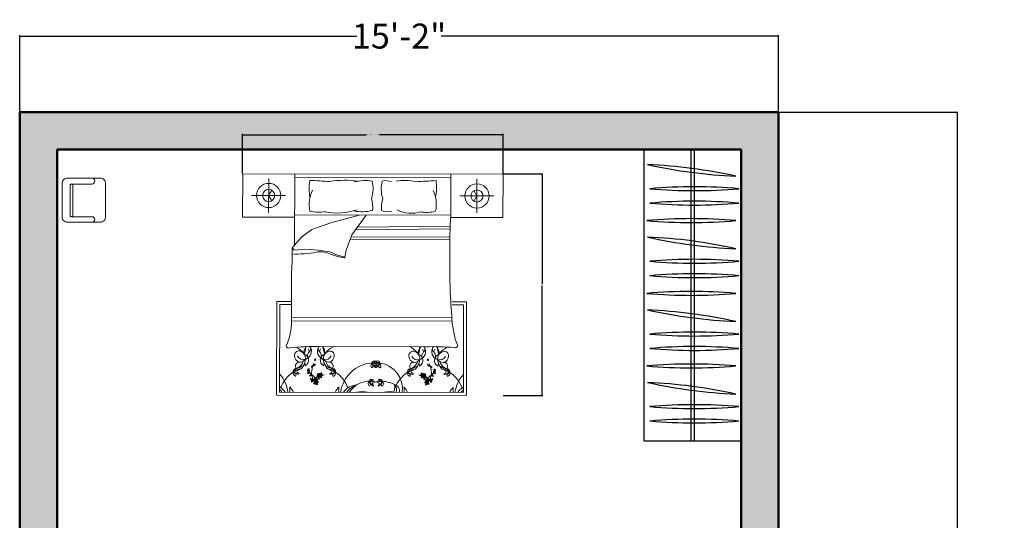
# Model space of a CAD drawing. Units: inches. Extents: x 3 to 485, y -522 to 42.
# Tile 6 of 6: x 249 to 485, y -84 to 36. Entities that reach past the tile are written whole.
import ezdxf

# ---------------------------------------------------------------- set-up
doc = ezdxf.new("R2010")
doc.units = ezdxf.units.IN
doc.header["$MEASUREMENT"] = 0
for name, color, linetype, lineweight in [('A-ANNO-DIMS', 2, 'Continuous', 18), ('A-FLOR-CASE', 8, 'Continuous', 25), ('A-FURN', 8, 'Continuous', 18), ('A-WALL', 7, 'Continuous', 50)]:
    doc.layers.add(name, color=color, linetype=linetype, lineweight=lineweight)
doc.layers.add('A-WALL-PATT', color=18, linetype='Continuous', lineweight=13, true_color=0x000000)
doc.styles.get("Standard").update_dxf_attribs({"font": 'arial.ttf'})
doc.dimstyles.get("Standard").update_dxf_attribs({"dimtxt": 0.18, "dimasz": 0.18, "dimexe": 0.18, "dimexo": 0.0625, "dimgap": 0.09, "dimtad": 0, "dimtih": 1, "dimtoh": 1, "dimdec": 0, "dimzin": 0, "dimdsep": 46, "dimlunit": 3, "dimtxsty": 'Standard', "dimcen": 0.09, "dimadec": 0, "dimazin": 0, "dimtfac": 1, "dimtdec": 0, "dimtofl": 0, "dimtmove": 0, "dimatfit": 3, "dimfxl": 1, "dimtolj": 1, "dimtzin": 0, "dimarcsym": 0})

# ---------------------------------------------------------------- blocks, each defined once
blk = doc.blocks.new('*D6')
at = {"layer": 'A-ANNO-DIMS', "color": 0, "lineweight": -2, "transparency": 16777216}
for p, q in [((248.79, 14.07), (248.79, 32.43)), ((248.97, 32.25), (329.68, 32.25)), ((430.61, 32.25), (349.9, 32.25)), ((430.79, 14.07), (430.79, 32.43))]:
    blk.add_line(p, q, dxfattribs=at)
at = {"layer": 'A-ANNO-DIMS', "color": 0, "transparency": 16777216}
for points in [[(248.97, 32.28), (248.97, 32.22), (248.79, 32.25)], [(430.61, 32.28), (430.61, 32.22), (430.79, 32.25)]]:
    blk.add_solid(points, dxfattribs=at)
at = {"layer": 'Defpoints', "color": 0, "transparency": 16777216}
for p in [(430.79, 32.25), (248.79, 14), (430.79, 14)]:
    blk.add_point(p, dxfattribs=at)
at = {"layer": 'A-ANNO-DIMS', "color": 0, "transparency": 16777216, "insert": (339.79, 32.25), "char_height": 6, "attachment_point": 5}
blk.add_mtext('\\A1;15\'-2"', dxfattribs=at)
blk = doc.blocks.new('*D7')
at = {"layer": 'A-ANNO-DIMS', "color": 0, "lineweight": -2, "transparency": 16777216}
for p, q in [((430.85, 14), (473.81, 14)), ((473.63, 13.82), (473.63, -230.89)), ((473.63, -481.82), (473.63, -237.1)), ((430.85, -482), (473.81, -482))]:
    blk.add_line(p, q, dxfattribs=at)
at = {"layer": 'A-ANNO-DIMS', "color": 0, "transparency": 16777216}
for points in [[(473.6, 13.82), (473.66, 13.82), (473.63, 14)], [(473.6, -481.82), (473.66, -481.82), (473.63, -482)]]:
    blk.add_solid(points, dxfattribs=at)
at = {"layer": 'Defpoints', "color": 0, "transparency": 16777216}
for p in [(430.79, 14), (430.79, -482), (473.63, -482)]:
    blk.add_point(p, dxfattribs=at)
at = {"layer": 'A-ANNO-DIMS', "color": 0, "transparency": 16777216, "insert": (473.63, -234), "char_height": 6, "attachment_point": 5}
blk.add_mtext('\\A1;41\'-4"', dxfattribs=at)
blk = doc.blocks.new('BED-DOUBLE-WITH-NIGHTSTANDS')
for p, q in [((53.23, 62.45), (53.09, 0)), ((48, 52.14), (48.02, 60.3)), ((0, 8.8), (0.1, 54.33)), ((0.1, 54.33), (22.6, 54.28)), ((43.93, 56.23), (52.09, 56.21)), ((0.82, 53.6), (0.73, 9.52)), ((21.87, 53.56), (0.82, 53.6)), ((21.87, 50.75), (21.87, 53.56)), ((22.6, 54.28), (22.59, 50.74)), ((17.83, 12.23), (17.92, 50.76)), ((18.61, 12.28), (18.7, 50.76)), ((34.9, 50.06), (35.41, 50.56)), ((35.15, 47.53), (34.9, 50.06)), ((35.41, 50.56), (38.06, 48.28)), ((53.2, 49.96), (36.06, 50)), ((43.33, 49.98), (43.25, 12.51)), ((52.32, 12.49), (52.4, 49.96)), ((7.14, 47.43), (7.85, 47.57)), ((34.89, 44.36), (35.15, 47.53)), ((38.06, 48.28), (39.83, 45.87)), ((39.83, 45.87), (41.46, 41.31)), ((7.13, 43.07), (7.84, 42.93)), ((11.71, 18.64), (11.77, 44)), ((34.51, 41.58), (34.89, 44.36)), ((33.74, 39.94), (34.51, 41.58)), ((41.46, 41.31), (43.3, 34.5)), ((33.23, 37.92), (33.74, 39.94)), ((34.88, 37.66), (33.23, 37.92)), ((38.54, 36.26), (34.88, 37.66)), ((37.41, 12.75), (37.36, 36.71)), ((38.05, 12.75), (38.01, 36.46)), ((43.3, 32.83), (38.54, 36.26)), ((40.02, 12.71), (39.75, 35.39)), ((40.66, 12.69), (40.39, 34.92)), ((7.08, 20.02), (7.79, 20.16)), ((7.07, 15.66), (7.78, 15.52)), ((21.78, 9.47), (21.78, 12.22)), ((22.51, 12.21), (22.5, 8.75)), ((0.73, 9.52), (21.78, 9.47)), ((47.91, 10.34), (47.89, 2.18)), ((22.5, 8.75), (0, 8.8)), ((43.82, 6.27), (51.98, 6.25))]:
    blk.add_line(p, q)
for points in [[(42.79, 49.99), (42.82, 62.48), (53.23, 62.45)], [(48.01, 56.22), (46.75, 55.49)], [(48.01, 56.22), (49.27, 55.49)], [(53.12, 12.49), (42.71, 12.51), (42.69, 0.02), (53.09, 0)], [(47.9, 6.26), (46.64, 6.99)], [(47.9, 6.26), (49.17, 6.98)]]:
    blk.add_lwpolyline(points)
for points in [[(29.69, 50.7, 0.001242), (17.84, 50.76, -0.127202), (11.94, 52.03)], [(51.64, 46.38, 0.074897), (47.56, 46.31, -0.472817)], [(47.3, 31.53, 0.14099), (51.46, 31.4, 0.235245)], [(47.29, 28.87, -0.14099), (51.46, 28.98, -0.235245)], [(51.57, 16.08, -0.074897), (47.49, 16.17, 0.472817)], [(19.1, 12.3, 0.056112), (15.67, 11.85, 0.095341), (12.35, 10.98)]]:
    blk.add_lwpolyline(points, format="xyb")
for centre, radius in [((48.01, 56.22), 2.91), ((48.01, 56.22), 1.46), ((3.2, 44.87), 0.159), ((4.87, 43.83), 0.159), ((4.82, 19.27), 0.159), ((3.14, 18.23), 0.159), ((47.9, 6.26), 2.91), ((47.9, 6.26), 1.46)]:
    blk.add_circle(centre, radius)
for centre, radius, start, end in [((-2.1, 57.02), 4.95, 306.1777, 316.3555), ((-1.36, 55.59), 3.97, 303.3358, 329.9857), ((-0.26, 59.68), 8.16, 277.6191, 311.7597), ((-1.1, 45.72), 8.16, 34.2606, 68.4649), ((11.98, 51.45), 0.576, 93.8541, 207.2153), ((-0.45, 53.36), 3.32, 292.4288, 318.8287), ((1.35, 62.44), 11.28, 267.2822, 273.526), ((5.45, 49.43), 0.904, 77.5856, 158.9128), ((4.96, 50.34), 0.681, 238.3374, 358.161), ((7.19, 48.96), 2.06, 138.7143, 177.8093), ((5.95, 49.72), 0.667, 117.5568, 223.6503), ((5.8, 49.66), 0.676, 2.8257, 103.6021), ((11.21, 51.54), 5.71, 192.3914, 207.0565), ((4.88, 49.27), 1.29, 345.3394, 54.1084), ((6.83, 51.04), 1.39, 211.2568, 255.171), ((7.09, 48.86), 0.937, 350.1381, 160.7429), ((9.5, 48.51), 1.49, 84.8189, 172.7598), ((9.65, 48.95), 1.05, 354.3597, 90.9279), ((-53.24, 44.88), 65.02, 359.2174, 5.5628), ((33.98, 107.83), 57.28, 265.7035, 271.4271), ((57.53, 49.44), 23.57, 177.326, 191.2133), ((5.23, 49.03), 0.101, 177.8093, 11.3575), ((5.28, 49.04), 0.0492, 11.3575, 127.815), ((5.53, 49.32), 0.0882, 223.6503, 159.5924), ((7.38, 49.09), 1.17, 175.8431, 254.1786), ((6.08, 49.06), 0.574, 333.8496, 53.1422), ((5.82, 47.83), 1.25, 6.0403, 51.4566), ((9.16, 50.72), 2.95, 211.1355, 251.5786), ((8.92, 50.74), 3.35, 236.1624, 266.3817), ((8.49, 48.2), 1.55, 209.7826, 343.0078), ((9.83, 48.77), 1.81, 182.2332, 233.9142), ((10.06, 47.93), 1.45, 111.456, 201.2962), ((8.87, 49.27), 1.88, 265.1674, 346.7951), ((9.14, 47.22), 0.388, 167.1782, 285.0212), ((10.18, 45.36), 2.41, 122.5752, 126.2186), ((10.64, 47.96), 1.99, 199.1563, 299.0492), ((11.32, 49.96), 2.59, 238.6959, 279.0295), ((10.18, 45.36), 2.41, 55.6591, 94.6045), ((7.39, 51.7), 4.73, 303.5412, 333.1738), ((11.08, 46.76), 0.752, 29.9034, 52.1991), ((2.9, 44.66), 0.263, 61.0937, 168.9144), ((3.07, 45.2), 0.314, 157.2827, 261.3127), ((2.9, 45.21), 0.158, 57.924, 135.5009), ((3.06, 45.11), 0.105, 172.7801, 277.0061), ((2.72, 44.92), 0.501, 14.6299, 57.924), ((3.42, 45.05), 0.217, 35.9787, 181.3022), ((3.43, 45.9), 0.178, 124.2279, 214.2664), ((3.69, 45.87), 0.414, 190.1798, 287.0699), ((3.29, 45.22), 0.219, 269.9386, 331.0248), ((3.48, 45.17), 0.25, 221.7153, 265.6618), ((3.81, 46.02), 0.481, 176.8442, 248.1654), ((7.25, 48.55), 4.65, 212.5525, 216.2487), ((3.48, 45.07), 0.156, 263.6267, 41.5794), ((3.44, 44.65), 0.265, 11.4378, 86.2391), ((3.65, 45.91), 0.184, 216.2487, 291.6289), ((5.27, 43.32), 2.59, 123.8774, 132.3658), ((2.6, 43), 2.77, 63.656, 68.1654), ((4.08, 45.13), 0.441, 128.1949, 208.6903), ((4.09, 45.78), 0.414, 122.6896, 187.2733), ((4.16, 45.16), 0.527, 207.5784, 254.2257), ((3.77, 45.61), 0.139, 289.2346, 111.6289), ((3.87, 45.61), 0.139, 221.7444, 44.1387), ((4.5, 45.2), 0.725, 157.1046, 228.9376), ((4.27, 45.72), 0.481, 109.354, 177.5569), ((4.25, 45.44), 0.427, 174.3285, 220.4929), ((1.82, 43.06), 3.11, 30.4181, 49.6921), ((4.01, 46.03), 0.178, 56.7377, 146.7762), ((4.1, 45.83), 0.184, 148.7585, 224.1387), ((3.54, 44.83), 0.513, 339.8782, 40.4929), ((7.92, 43.52), 4.65, 145.0623, 148.7585), ((5.27, 43.32), 2.59, 94.6301, 119.0782), ((10.78, 39.58), 8.53, 132.1153, 142.0485), ((6.49, 46.38), 1.76, 178.2005, 187.0043), ((4.59, 46.14), 0.328, 11.1997, 64.3362), ((5.7, 46.61), 0.987, 190.1329, 210.5301), ((5.04, 46.21), 0.3, 188.2173, 274.161), ((5.3, 46.37), 0.523, 210.5301, 242.5082), ((5.7, 46.82), 1, 218.0842, 226.1812), ((4.95, 45.98), 0.127, 325.6398, 67.3157), ((1.01, 50.24), 5.93, 313.0282, 321.92), ((5.39, 40.75), 5.17, 73.4583, 93.7018), ((5.37, 46.67), 0.122, 142.3478, 264.9271), ((5.53, 46.7), 0.263, 127.6362, 168.9144), ((5.39, 46.92), 0.37, 264.9271, 338.2359), ((5.88, 46.41), 0.483, 113.3017, 137.4845), ((5.82, 46.91), 0.159, 183.1509, 356.5973), ((5.94, 46.62), 0.26, 139.663, 227.5532), ((5.85, 46.53), 0.137, 227.5532, 350.2228), ((5.32, 46.63), 0.521, 352.9593, 15.5912), ((5.67, 46.57), 0.329, 350.2228, 43.5279), ((6.28, 46.9), 0.382, 198.6004, 262.3773), ((5.97, 46.73), 0.152, 0.9822, 91.7416), ((6.07, 46.69), 0.265, 11.4378, 52.5099), ((6.26, 46.64), 0.123, 255.1097, 54.7989), ((8.59, 46), 1.76, 178.2005, 187.0043), ((6.69, 45.76), 0.328, 11.1997, 64.3362), ((7.8, 46.23), 0.987, 190.1329, 210.5301), ((7.14, 45.83), 0.3, 188.2173, 274.161), ((7.4, 46), 0.523, 210.5301, 242.5082), ((7.8, 46.44), 1, 218.0842, 226.1812), ((7.05, 45.6), 0.127, 325.6398, 67.3157), ((7.41, 45.37), 0.3, 147.4073, 233.3509), ((7.68, 45.52), 0.523, 179.06, 211.0381), ((7.17, 45.41), 0.127, 354.2525, 95.9284), ((5.39, 40.75), 5.17, 62.8773, 69.7682), ((8.08, 45.76), 0.987, 211.0381, 231.4353), ((8.25, 46.56), 1.76, 234.5639, 243.3677), ((8.27, 45.66), 1, 195.387, 203.484), ((7.14, 45.01), 0.328, 357.232, 50.3685), ((8.55, 45.07), 0.12, 12.5792, 190.3125), ((8.62, 45.08), 0.196, 190.3125, 10.2877), ((9.57, 45.61), 1.28, 41.4394, 105.0212), ((10.28, 48.26), 1.8, 277.3101, 299.789), ((11.23, 47.07), 0.935, 221.4394, 293.7095), ((11.08, 46.76), 0.752, 314.3258, 333.4321), ((52.37, 44.15), 8.37, 164.978, 190.911), ((45.9, 38.43), 8.05, 65.0057, 101.6324), ((645.92, 10.65), 595.35, 176.55931, 177.02387), ((2.74, 44.63), 0.122, 142.3478, 264.9271), ((2.76, 44.88), 0.37, 264.9271, 338.2359), ((3.25, 44.37), 0.483, 113.3017, 137.4845), ((3.31, 44.59), 0.26, 139.663, 227.5532), ((3.23, 44.5), 0.137, 227.5532, 350.2228), ((2.7, 44.59), 0.521, 352.9593, 15.5912), ((3.04, 44.53), 0.329, 350.2228, 43.5279), ((3.65, 44.87), 0.382, 198.6004, 262.3773), ((3.35, 44.69), 0.152, 0.9822, 91.7416), ((3.63, 44.61), 0.123, 255.1097, 54.7989), ((3.82, 44.86), 0.725, 270.1521, 341.9851), ((4.3, 43.95), 0.513, 98.5968, 159.2116), ((4.05, 44.61), 0.527, 244.864, 291.5114), ((4.16, 44.88), 0.427, 278.5968, 324.7613), ((4.09, 44.54), 0.441, 290.3994, 358.4116), ((4.41, 43.59), 0.122, 142.3478, 264.9271), ((4.57, 43.61), 0.263, 61.0937, 168.9144), ((4.44, 43.84), 0.37, 264.9271, 338.2359), ((4.75, 44.15), 0.314, 157.2827, 261.3127), ((4.57, 44.17), 0.158, 57.924, 135.5009), ((4.95, 44.66), 0.441, 182.724, 265.9967), ((4.78, 44.97), 0.427, 231.6348, 277.7993), ((5.11, 45.05), 0.725, 214.411, 286.244), ((4.92, 43.33), 0.483, 113.3017, 137.4845), ((4.74, 44.07), 0.105, 172.7801, 277.0061), ((4.39, 43.87), 0.501, 14.6299, 57.924), ((1.82, 43.06), 3.11, 22.9242, 23.7218), ((4.99, 43.54), 0.26, 139.663, 227.5532), ((4.9, 43.45), 0.137, 227.5532, 350.2228), ((4.9, 44.04), 0.513, 37.1845, 97.7993), ((5.09, 44.01), 0.217, 35.9787, 181.3022), ((4.37, 43.55), 0.521, 352.9593, 15.5912), ((4.96, 44.75), 0.527, 264.8847, 311.5321), ((1.82, 43.06), 3.11, 356.9812, 4.6326), ((4.71, 43.48), 0.329, 350.2228, 43.5279), ((5.32, 43.82), 0.382, 198.6004, 262.3773), ((4.97, 44.18), 0.219, 269.9386, 331.0248), ((5.15, 44.12), 0.25, 221.7153, 265.6618), ((5.02, 43.64), 0.152, 0.9822, 91.7416), ((5.15, 44.03), 0.156, 263.6267, 41.5794), ((5.12, 43.61), 0.265, 11.4378, 86.2391), ((5.3, 43.56), 0.123, 255.1097, 54.7989), ((7.36, 41.41), 1.17, 105.5696, 183.9051), ((5.81, 42.68), 1.25, 308.2916, 353.7079), ((9.14, 39.78), 2.95, 108.1696, 148.6127), ((8.9, 39.75), 3.35, 93.3665, 123.5858), ((8.48, 42.29), 1.55, 16.7404, 149.9656), ((9.81, 41.72), 1.81, 125.834, 177.515), ((10.05, 42.56), 1.45, 158.4519, 248.2922), ((8.85, 41.22), 1.88, 12.9531, 94.5808), ((9.13, 43.27), 0.388, 74.727, 192.57), ((10.63, 42.53), 1.99, 60.699, 160.5919), ((10.18, 45.13), 2.41, 233.5296, 237.173), ((9.57, 44.88), 1.28, 254.727, 318.3088), ((11.3, 40.52), 2.59, 79.5874, 121.0523), ((10.18, 45.13), 2.41, 265.1437, 304.089), ((7.36, 38.8), 4.73, 21.3682, 56.207), ((10.27, 42.23), 1.8, 59.9592, 82.4381), ((11.22, 43.41), 0.935, 66.0387, 138.3088), ((11.08, 43.73), 0.752, 307.5491, 336.5885), ((11.08, 43.73), 0.752, 23.1031, 45.4224), ((29.42, 43.87), 5.08, 336.1357, 11.2133), ((58.3, 39.73), 14.52, 167.9138, 199.1356), ((-0.49, 37.18), 3.32, 40.9195, 67.3194), ((-1.1, 44.81), 8.16, 291.2833, 325.4876), ((4.94, 40.17), 0.681, 1.5872, 121.4108), ((5.43, 41.08), 0.904, 200.8354, 282.1626), ((5.21, 41.48), 0.101, 348.3907, 181.9389), ((7.17, 41.55), 2.06, 181.9389, 221.0339), ((5.26, 41.47), 0.0492, 231.9332, 348.3907), ((5.93, 40.78), 0.667, 136.0979, 242.1914), ((5.55, 41.17), 0.0532, 200.1408, 136.1012), ((4.87, 41.24), 1.29, 305.6398, 14.4087), ((11.19, 38.94), 5.71, 152.6917, 167.3568), ((5.78, 40.85), 0.676, 256.1461, 356.9225), ((6.81, 39.46), 1.39, 104.5772, 148.4914), ((7.08, 41.64), 0.937, 199.0053, 9.6101), ((6.06, 41.45), 0.574, 306.606, 25.8985), ((9.48, 41.98), 1.49, 186.9883, 274.9292), ((9.63, 41.55), 1.05, 268.8203, 5.3885), ((56.83, 33.53), 24.22, 159.9935, 169.2124), ((29.02, 37.87), 22.65, 352.0937, 9.3711), ((1.28, 28.09), 11.28, 86.2222, 92.466), ((-0.33, 30.86), 8.16, 4.3364, 82.1291), ((-1.41, 34.95), 3.97, 1.1461, 56.4124), ((33.18, 38.06), 0.151, 178.7364, 289.6277), ((-2.15, 33.52), 4.95, 17.7245, 53.5705), ((-3.55, 30.92), 7.37, 33.8864, 53.9271), ((55.12, 33.86), 11.01, 169.7358, 193.4979), ((40.46, 33.06), 11.13, 351.399, 13.8341), ((-3.51, 33.77), 4.48, 343.4172, 16.8943), ((-4.69, 31.49), 8.16, 4.3364, 27.2887), ((-5.82, 32), 6.63, 4.2528, 5.5098), ((-10.38, 28.52), 11.85, 19.5958, 19.7769), ((2.83, 31.44), 0.904, 47.6614, 128.9886), ((2.86, 32.47), 0.681, 208.4132, 328.2368), ((2.44, 31.2), 0.101, 147.8851, 341.4333), ((4.1, 30.16), 2.06, 108.79, 147.8851), ((2.49, 31.18), 0.0492, 341.4333, 97.8908), ((3.41, 31.44), 0.667, 87.6326, 193.7261), ((2.85, 31.31), 0.0882, 193.7261, 129.7986), ((8.88, 30.39), 5.71, 162.4671, 177.1323), ((2.26, 31.58), 1.29, 315.4152, 24.1842), ((4.83, 32.14), 1.39, 181.3326, 225.2468), ((3.25, 31.46), 0.676, 332.9015, 73.6778), ((7.2, 30.81), 0.904, 47.6614, 128.9886), ((7.23, 31.83), 0.681, 208.4132, 328.2368), ((8.47, 29.52), 2.06, 108.79, 147.8851), ((7.78, 30.81), 0.667, 87.6326, 193.7261), ((7.22, 30.67), 0.0882, 193.7261, 129.7986), ((6.63, 30.95), 1.29, 315.4152, 24.1842), ((13.25, 29.76), 5.71, 162.4671, 177.1323), ((6.63, 30.06), 1.29, 335.564, 44.333), ((13.25, 31.23), 5.71, 182.6159, 197.2811), ((7.62, 30.83), 0.676, 332.9015, 73.6778), ((9.2, 31.51), 1.39, 181.3326, 225.2468), ((45.23, 38.9), 7.65, 263.887, 285.7034), ((1.56, 30.44), 6.31, 262.7377, 351.6938), ((-3.52, 27.29), 4.48, 342.8539, 16.331), ((-5.83, 29.07), 6.63, 354.2384, 355.4954), ((-10.37, 32.57), 11.85, 339.9713, 340.1524), ((2.85, 28.56), 0.681, 31.5114, 151.335), ((2.83, 29.59), 0.904, 230.7596, 312.0868), ((2.44, 29.83), 0.101, 18.3149, 211.8631), ((4.1, 30.87), 2.06, 211.8631, 250.9581), ((2.49, 29.85), 0.0492, 261.8574, 18.3149), ((-4.7, 29.57), 8.16, 332.4595, 355.4118), ((3.41, 29.58), 0.667, 166.0221, 272.1156), ((2.88, 29.73), 0.0532, 230.065, 165.895), ((8.88, 30.61), 5.71, 182.6159, 197.2811), ((2.26, 29.45), 1.29, 335.564, 44.333), ((4.82, 28.88), 1.39, 134.5014, 178.4156), ((3.24, 29.57), 0.676, 286.0703, 26.8467), ((7.22, 29.18), 0.681, 31.5114, 151.335), ((7.2, 30.2), 0.904, 230.7596, 312.0868), ((6.81, 30.57), 0.101, 147.8851, 341.4333), ((6.81, 30.45), 0.101, 18.3149, 211.8631), ((8.47, 31.48), 2.06, 211.8631, 250.9581), ((6.86, 30.55), 0.0492, 341.4333, 97.8908), ((6.86, 30.46), 0.0492, 261.8574, 18.3149), ((7.78, 30.2), 0.667, 166.0221, 272.1156), ((7.25, 30.35), 0.0532, 230.065, 165.895), ((7.61, 30.18), 0.676, 286.0703, 26.8467), ((9.19, 29.49), 1.39, 134.5014, 178.4156), ((47.41, 27.72), 3.31, 154.8924, 198.4148), ((45.19, 21.51), 7.65, 74.0448, 95.8612), ((48.49, 28.13), 3.09, 333.2178, 15.9767), ((2.13, 29.63), 3.65, 247.9911, 276.4936), ((1.11, 26.28), 1.46, 256.2639, 348.9479), ((1.31, 27.38), 1.85, 252.735, 311.779), ((1.29, 35.03), 11.28, 267.2822, 273.526), ((-0.51, 25.95), 3.32, 292.4288, 318.8287), ((-1.16, 18.31), 8.16, 34.2606, 68.4649), ((51.7, 21.92), 7.95, 153.7502, 196.0487), ((40.66, 23.52), 10.98, 346.2168, 11.0582), ((5.39, 22.02), 0.904, 77.5856, 158.9128), ((4.9, 22.93), 0.681, 238.3374, 358.161), ((7.13, 21.54), 2.06, 138.7143, 177.8093), ((5.17, 21.62), 0.101, 177.8093, 11.3575), ((5.22, 21.63), 0.0492, 11.3575, 127.815), ((5.89, 22.31), 0.667, 117.5568, 223.6503), ((5.47, 21.91), 0.0882, 223.6503, 159.5924), ((5.74, 22.25), 0.676, 2.8257, 103.6021), ((6.77, 23.63), 1.39, 211.2568, 255.171), ((4.82, 21.86), 1.29, 345.3394, 54.1084), ((11.15, 24.13), 5.71, 192.3914, 207.0565), ((7.03, 21.45), 0.937, 350.1381, 160.7429), ((7.32, 21.68), 1.17, 175.8431, 254.1786), ((6.02, 21.65), 0.574, 333.8496, 53.1422), ((5.76, 20.42), 1.25, 6.0403, 51.4566), ((9.1, 23.31), 2.95, 211.1355, 251.5786), ((9.44, 21.1), 1.49, 84.8189, 172.7598), ((9.77, 21.36), 1.81, 182.2332, 233.9142), ((10, 20.52), 1.45, 111.456, 201.2962), ((8.81, 21.86), 1.88, 265.1674, 346.7951), ((9.59, 21.54), 1.05, 354.3597, 90.9279), ((7.33, 24.29), 4.73, 303.5412, 338.38), ((3.99, 18.49), 0.527, 68.2368, 114.8842), ((3.76, 18.24), 0.725, 17.763, 89.5961), ((4.25, 19.15), 0.513, 200.5366, 261.1514), ((4.03, 18.57), 0.441, 1.3366, 69.3488), ((4.36, 19.51), 0.122, 94.8211, 217.4004), ((4.52, 19.49), 0.263, 190.8338, 298.6545), ((4.38, 19.27), 0.37, 21.5123, 94.8211), ((4.69, 18.95), 0.314, 98.4355, 202.4655), ((4.87, 19.77), 0.483, 222.2637, 246.4465), ((4.68, 19.04), 0.105, 82.7421, 186.9681), ((4.34, 19.23), 0.501, 301.8242, 345.1183), ((4.93, 19.56), 0.26, 132.1949, 220.0852), ((4.85, 19.65), 0.137, 9.5254, 132.1949), ((4.32, 19.56), 0.521, 344.157, 6.7889), ((5.04, 19.1), 0.217, 178.446, 323.7695), ((1.77, 20.05), 3.11, 355.1156, 2.767), ((4.66, 19.62), 0.329, 316.2203, 9.5254), ((5.27, 19.28), 0.382, 97.3709, 161.1478), ((5.1, 18.98), 0.25, 94.0864, 138.0328), ((4.91, 18.92), 0.219, 28.7234, 89.8096), ((4.97, 19.46), 0.152, 268.0066, 358.766), ((5.06, 19.49), 0.265, 273.5091, 348.3104), ((5.1, 19.07), 0.156, 318.1687, 96.1215), ((5.25, 19.54), 0.123, 304.9493, 104.6385), ((8.86, 23.33), 3.35, 236.1624, 266.3817), ((8.43, 20.79), 1.55, 209.7826, 343.0078), ((9.08, 19.81), 0.388, 167.1782, 285.0212), ((10.12, 17.95), 2.41, 122.5752, 126.2186), ((10.58, 20.55), 1.99, 199.1563, 299.0492), ((9.51, 18.2), 1.28, 41.4394, 105.0212), ((11.26, 22.55), 2.59, 238.6959, 280.1608), ((10.12, 17.95), 2.41, 55.6591, 94.6045), ((10.22, 20.85), 1.8, 277.3101, 299.789), ((11.17, 19.66), 0.935, 221.4394, 293.7095), ((11.02, 19.35), 0.752, 23.1597, 52.1991), ((11.02, 19.35), 0.752, 314.3258, 336.5885), ((52.31, 18.31), 8.37, 168.8372, 194.7702), ((646, 49.2), 595.35, 182.72432, 183.18889), ((2.68, 18.48), 0.122, 94.8211, 217.4004), ((2.84, 18.45), 0.263, 190.8338, 298.6545), ((2.7, 18.23), 0.37, 21.5123, 94.8211), ((3.01, 17.91), 0.314, 98.4355, 202.4655), ((2.84, 17.9), 0.158, 224.2473, 301.8242), ((3.19, 18.73), 0.483, 222.2637, 246.4465), ((3, 18), 0.105, 82.7421, 186.9681), ((2.66, 18.19), 0.501, 301.8242, 345.1183), ((3.25, 18.52), 0.26, 132.1949, 220.0852), ((3.17, 18.61), 0.137, 9.5254, 132.1949), ((2.64, 18.52), 0.521, 344.157, 6.7889), ((3.36, 18.06), 0.217, 178.446, 323.7695), ((3.37, 17.21), 0.178, 145.4818, 235.5203), ((2.98, 18.58), 0.329, 316.2203, 9.5254), ((3.63, 17.23), 0.414, 72.6783, 169.5684), ((3.59, 18.24), 0.382, 97.3709, 161.1478), ((3.42, 17.94), 0.25, 94.0864, 138.0328), ((3.23, 17.89), 0.219, 28.7234, 89.8096), ((3.75, 17.09), 0.481, 111.5828, 182.904), ((7.17, 14.54), 4.65, 143.4995, 147.1957), ((3.29, 18.42), 0.152, 268.0066, 358.766), ((3.38, 18.45), 0.265, 273.5091, 348.3104), ((3.42, 18.03), 0.156, 318.1687, 96.1215), ((3.58, 17.2), 0.184, 68.1193, 143.4995), ((5.22, 19.78), 2.59, 227.3824, 235.8708), ((3.57, 18.5), 0.123, 304.9493, 104.6385), ((2.55, 20.11), 2.77, 291.5828, 296.0922), ((4.02, 17.97), 0.441, 151.0579, 231.5533), ((4.02, 17.33), 0.414, 172.4749, 237.0586), ((4.11, 17.94), 0.527, 105.5225, 152.1698), ((3.7, 17.5), 0.139, 248.1193, 70.5136), ((4.44, 17.9), 0.725, 130.8106, 202.6436), ((3.81, 17.5), 0.139, 315.6095, 138.0038), ((4.21, 17.38), 0.481, 182.1913, 250.3942), ((1.77, 20.05), 3.11, 310.0561, 329.3301), ((4.19, 17.66), 0.427, 139.2553, 185.4197), ((3.95, 17.08), 0.178, 212.972, 303.0105), ((4.04, 17.27), 0.184, 135.6095, 210.9897), ((3.48, 18.28), 0.513, 319.2553, 19.87), ((7.86, 19.57), 4.65, 210.9897, 214.6859), ((5.22, 19.78), 2.59, 240.67, 265.1181), ((10.75, 23.5), 8.53, 217.6997, 227.6329), ((4.1, 18.22), 0.427, 34.9869, 81.1514), ((4.52, 18.94), 0.158, 224.2473, 301.8242), ((4.89, 18.44), 0.441, 93.7515, 177.0242), ((5.05, 18.05), 0.725, 73.5042, 145.3372), ((4.72, 18.13), 0.427, 81.9489, 128.1134), ((1.77, 20.05), 3.11, 336.0264, 336.824), ((5.63, 16.49), 0.987, 149.2181, 169.6153), ((6.42, 16.72), 1.76, 172.7439, 181.5477), ((4.52, 16.96), 0.328, 295.412, 348.5485), ((4.97, 16.89), 0.3, 85.5872, 171.5309), ((4.85, 19.06), 0.513, 261.9489, 322.5636), ((5.24, 16.73), 0.523, 117.24, 149.2181), ((5.63, 16.28), 1, 133.567, 141.664), ((4.9, 18.36), 0.527, 48.2161, 94.8635), ((4.89, 17.12), 0.127, 292.4324, 34.1083), ((5.35, 22.35), 5.17, 266.0464, 286.2899), ((0.93, 12.88), 5.93, 37.8282, 46.72), ((5.3, 16.43), 0.122, 94.8211, 217.4004), ((5.32, 16.18), 0.37, 21.5123, 94.8211), ((5.87, 16.47), 0.26, 132.1949, 220.0852), ((5.79, 16.56), 0.137, 9.5254, 132.1949), ((5.26, 16.47), 0.521, 344.157, 6.7889), ((5.6, 16.53), 0.329, 316.2203, 9.5254), ((6.21, 16.19), 0.382, 97.3709, 161.1478), ((6.19, 16.45), 0.123, 304.9493, 104.6385), ((8.53, 17.08), 1.76, 172.7439, 181.5477), ((7.74, 16.86), 0.987, 149.2181, 169.6153), ((6.62, 17.33), 0.328, 295.412, 348.5485), ((7.08, 17.26), 0.3, 85.5872, 171.5309), ((7.34, 17.09), 0.523, 117.24, 149.2181), ((7.73, 16.64), 1, 133.567, 141.664), ((6.99, 17.49), 0.127, 292.4324, 34.1083), ((7.35, 17.72), 0.3, 126.3973, 212.3409), ((7.62, 17.57), 0.523, 148.7101, 180.6882), ((7.11, 17.69), 0.127, 263.8198, 5.4957), ((5.35, 22.35), 5.17, 289.98, 296.8709), ((8.02, 17.33), 0.987, 128.3129, 148.7101), ((8.19, 16.52), 1.76, 116.3805, 125.1843), ((8.2, 17.43), 1, 156.2642, 164.3612), ((7.08, 18.09), 0.328, 309.3797, 2.5162), ((8.56, 18), 0.196, 349.4605, 169.4356), ((8.49, 18.02), 0.12, 169.4356, 347.169), ((10.57, 15.12), 1.99, 60.699, 160.5919), ((9.51, 17.47), 1.28, 254.727, 318.3088), ((10.21, 14.82), 1.8, 59.9592, 82.4381), ((11.16, 16), 0.935, 66.0387, 138.3088), ((-49.04, 16.86), 60.77, 355.1143, 1.6776), ((11.01, 16.32), 0.752, 16.5084, 45.4224), ((45.87, 24.05), 8.05, 258.1158, 294.7425), ((5.15, 14.07), 0.101, 348.3907, 181.9389), ((5.46, 16.4), 0.263, 190.8338, 232.112), ((5.81, 16.69), 0.483, 222.2637, 246.4465), ((5.75, 16.19), 0.159, 3.1509, 176.5973), ((5.91, 16.37), 0.152, 268.0066, 358.766), ((7.3, 14), 1.17, 105.5696, 183.9051), ((7.02, 14.23), 0.937, 199.0053, 9.6101), ((6, 16.41), 0.265, 307.2383, 348.3104), ((6, 14.04), 0.574, 306.606, 25.8985), ((5.75, 15.27), 1.25, 308.2916, 353.7079), ((9.08, 12.37), 2.95, 108.1696, 148.6127), ((8.84, 12.34), 3.35, 93.3665, 123.5858), ((8.42, 14.88), 1.55, 16.7404, 149.9656), ((9.75, 14.31), 1.81, 125.834, 177.515), ((9.42, 14.57), 1.49, 186.9883, 274.9292), ((9.99, 15.15), 1.45, 158.4519, 248.2922), ((8.79, 13.81), 1.88, 12.9531, 94.5808), ((9.07, 15.86), 0.388, 74.727, 192.57), ((10.12, 17.72), 2.41, 233.5296, 237.173), ((9.57, 14.14), 1.05, 268.8203, 5.3885), ((11.24, 13.11), 2.59, 79.1231, 121.0523), ((10.12, 17.72), 2.41, 265.1437, 304.089), ((7.3, 11.39), 4.73, 23.5194, 56.207), ((11.01, 16.32), 0.752, 307.5491, 342.4555), ((-0.55, 9.77), 3.32, 40.9195, 67.3194), ((1.22, 0.68), 11.28, 86.2222, 92.466), ((-1.16, 17.4), 8.16, 291.2833, 325.4876), ((4.88, 12.76), 0.681, 1.5872, 121.4108), ((5.37, 13.67), 0.904, 200.8354, 282.1626), ((7.11, 14.14), 2.06, 181.9389, 221.0339), ((5.2, 14.06), 0.0492, 231.9332, 348.3907), ((5.87, 13.37), 0.667, 136.0979, 242.1914), ((5.49, 13.76), 0.0532, 200.1408, 136.1012), ((11.12, 11.53), 5.71, 152.6917, 167.3568), ((4.81, 13.83), 1.29, 305.6398, 14.4087), ((6.75, 12.05), 1.39, 104.5772, 148.4914), ((5.72, 13.44), 0.676, 256.1461, 356.9225), ((31.22, -133.58), 146.38, 88.9886, 94.7476), ((35.37, -99.43), 112.22, 85.9741, 90.8023), ((-0.39, 3.45), 8.16, 47.9885, 82.1291), ((-1.47, 7.54), 3.97, 29.7625, 56.4124), ((-2.21, 6.11), 4.95, 43.3927, 53.5705), ((12.04, 11.46), 0.569, 156.396, 303.7005)]:
    blk.add_arc(centre, radius, start, end)
blk = doc.blocks.new('*D20')
at = {"layer": 'A-ANNO-DIMS', "color": 0, "lineweight": -2, "transparency": 16777216}
for p, q in [((302.24, -0.73), (302.24, 8.76)), ((302.42, 8.58), (331.85, 8.58)), ((364.54, 8.58), (335.12, 8.58)), ((364.72, -0.73), (364.72, 8.76))]:
    blk.add_line(p, q, dxfattribs=at)
at = {"layer": 'A-ANNO-DIMS', "color": 0, "transparency": 16777216}
for points in [[(302.42, 8.61), (302.42, 8.55), (302.24, 8.58)], [(364.54, 8.61), (364.54, 8.55), (364.72, 8.58)]]:
    blk.add_solid(points, dxfattribs=at)
at = {"layer": 'Defpoints', "color": 0, "transparency": 16777216}
for p in [(302.24, 8.58), (302.24, -0.79), (364.72, -0.79)]:
    blk.add_point(p, dxfattribs=at)
at = {"layer": 'A-ANNO-DIMS', "color": 0, "transparency": 16777216, "insert": (333.48, 8.58), "char_height": 0.18, "attachment_point": 5}
blk.add_mtext('\\A1;BED GROUP 5\'-2 1/2" TYP.', dxfattribs=at)
blk = doc.blocks.new('*D21')
at = {"layer": 'A-ANNO-DIMS', "color": 0, "lineweight": -2, "transparency": 16777216}
for p, q in [((364.78, -0.79), (374.27, -0.79)), ((374.09, -0.97), (374.09, -27.22)), ((374.09, -53.84), (374.09, -27.59)), ((364.78, -54.02), (374.27, -54.02))]:
    blk.add_line(p, q, dxfattribs=at)
at = {"layer": 'A-ANNO-DIMS', "color": 0, "transparency": 16777216}
for points in [[(374.06, -0.97), (374.12, -0.97), (374.09, -0.79)], [(374.06, -53.84), (374.12, -53.84), (374.09, -54.02)]]:
    blk.add_solid(points, dxfattribs=at)
at = {"layer": 'Defpoints', "color": 0, "transparency": 16777216}
for p in [(364.72, -0.79), (374.09, -0.79), (364.72, -54.02)]:
    blk.add_point(p, dxfattribs=at)
at = {"layer": 'A-ANNO-DIMS', "color": 0, "transparency": 16777216, "insert": (374.09, -27.41), "char_height": 0.18, "attachment_point": 5}
blk.add_mtext('\\A1;4\'-5" TYP.', dxfattribs=at)

msp = doc.modelspace()

# ---------------------------------------------------------------- hatches: boundary and pattern name
at = {"layer": 'A-WALL-PATT'}
h = msp.add_hatch(color=256, dxfattribs=at)
h.dxf.hatch_style = 1
h.paths.add_polyline_path([(257.79, 5), (421.79, 5), (421.79, -482), (430.79, -482), (430.79, 14), (248.79, 14), (248.79, -482), (257.79, -482), (257.79, -393), (311.15, -393), (311.15, -388.5), (257.79, -388.5), (257.79, -268.5), (392.64, -268.5), (392.64, -264), (257.79, -264)])
h.paths.add_polyline_path([(358.77, -482), (358.77, -473), (298.77, -473), (298.77, -482)], flags=17)
h.paths.add_polyline_path([(298.14, -167.5), (298.14, -143.5), (293.64, -143.5), (293.64, -167.5), (293.64, -172), (392.64, -172), (392.64, -167.5), (392.64, -119.5), (388.14, -119.5), (388.14, -167.5)], flags=17)
h.paths.add_polyline_path([(362.14, -119.5), (362.14, -115), (293.64, -115), (293.64, -119.5)], flags=17)

# ---------------------------------------------------------------- linework, layer by layer
at = {"layer": 'A-FLOR-CASE'}
for p, q in [((398.5, 5), (398.5, -64.88)), ((398.5, 5), (421.79, 5)), ((409.76, 5), (409.76, -64.88)), ((410.53, 5), (410.53, -64.88)), ((421.79, 5), (421.79, -64.88)), ((398.5, -64.88), (421.79, -64.88))]:
    msp.add_line(p, q, dxfattribs=at)
for centre, start, end in [((425.88, 121.07), 257.508, 267.5023), ((394.03, -121.03), 77.508, 87.5023), ((410.61, -126.48), 85.0028, 94.9972), ((410.61, 117.71), 265.0028, 274.9972), ((410.61, -129.94), 85.0028, 94.9972), ((410.61, 114.25), 265.0028, 274.9972), ((409.86, -134.13), 85.0028, 94.9972), ((409.86, 110.06), 265.0028, 274.9972), ((425.88, 103.66), 257.508, 267.5023), ((394.03, -138.44), 77.508, 87.5023), ((410.61, -143.89), 85.0028, 94.9972), ((410.61, 100.3), 265.0028, 274.9972), ((410.61, -147.35), 85.0028, 94.9972), ((410.61, 96.84), 265.0028, 274.9972), ((409.86, -151.61), 85.0028, 94.9972), ((409.86, 92.58), 265.0028, 274.9972), ((394.03, -155.92), 77.508, 87.5023), ((425.88, 86.19), 257.508, 267.5023), ((410.61, -161.37), 85.0028, 94.9972), ((410.61, 82.82), 265.0028, 274.9972), ((410.61, -164.82), 85.0028, 94.9972), ((410.61, 79.37), 265.0028, 274.9972), ((409.86, -169.02), 85.0028, 94.9972), ((409.86, 75.17), 265.0028, 274.9972), ((394.03, -173.33), 77.508, 87.5023), ((425.88, 68.78), 257.508, 267.5023), ((410.61, -178.78), 85.0028, 94.9972), ((410.61, 65.41), 265.0028, 274.9972), ((410.61, -182.23), 85.0028, 94.9972), ((410.61, 61.96), 265.0028, 274.9972)]:
    msp.add_arc(centre, 122.56, start, end, dxfattribs=at)
at = {"layer": 'A-FURN', "ltscale": 0.03}
msp.add_lwpolyline([(258.95, -11.1), (258.95, -11.1, 0.414214), (260.26, -12.41), (268.09, -12.41, 0.414214), (269.4, -11.1), (269.4, -11.1), (269.4, -3.14, 0.414214), (268.09, -1.83), (260.26, -1.83, 0.414214), (258.95, -3.14)], format="xyb", close=True, dxfattribs=at)
at = {"layer": 'A-FURN'}
for points in [[(266.13, -1.83, -0.414214), (266.79, -2.48), (266.79, -2.61, -0.414214), (266.13, -3.27), (265.12, -3.27)], [(261.56, -6.38), (261.56, -3.53, 0.414214), (261.3, -3.27), (261.17, -3.27, 0.414214), (260.91, -3.53)], [(260.91, -3.53), (260.91, -5.73, 0.414214)], [(260.91, -5.73), (260.91, -10.84, 0.414214), (261.17, -11.1), (261.3, -11.1, 0.414214), (261.56, -10.84), (261.56, -6.38, 0.414214)], [(261.3, -11.1), (266.13, -11.1, -0.414214), (266.79, -11.75), (266.79, -11.75, -0.414214), (266.13, -12.41)]]:
    msp.add_lwpolyline(points, format="xyb", dxfattribs=at)
for points in [[(265.12, -3.27), (260.91, -3.27), (260.91, -5.73)], [(260.91, -5.73), (260.91, -11.03)]]:
    msp.add_lwpolyline(points, dxfattribs=at)
at = {"layer": 'A-WALL'}
for p, q in [((248.79, 14), (248.79, -482)), ((248.79, 14), (430.79, 14)), ((430.79, 14), (430.79, -482)), ((257.79, 5), (257.79, -264)), ((257.79, 5), (421.79, 5)), ((421.79, 5), (421.79, -482))]:
    msp.add_line(p, q, dxfattribs=at)

# ---------------------------------------------------------------- block references
at = {"layer": 'A-FURN', "rotation": 89.99999999999994}
msp.add_blockref('BED-DOUBLE-WITH-NIGHTSTANDS', (364.72, -54.02), dxfattribs=at)

# ---------------------------------------------------------------- dimensions: what is measured, and where the dimension line sits
at = {"layer": 'A-ANNO-DIMS'}
dim = msp.add_linear_dim(base=(430.79, 32.25), p1=(248.79, 14), p2=(430.79, 14), dimstyle='Standard', override={"dimtxt": 6, "dimclrd": 0, "dimclre": 0, "dimclrt": 0}, dxfattribs=at)
dim.commit()
dim.dimension.update_dxf_attribs({"geometry": '*D6', "text_midpoint": (339.79, 32.25)})
dim = msp.add_linear_dim(base=(473.63, -482), p1=(430.79, 14), p2=(430.79, -482), angle=90, dimstyle='Standard', override={"dimtxt": 6, "dimclrd": 0, "dimclre": 0, "dimclrt": 0}, dxfattribs=at)
dim.commit()
dim.dimension.update_dxf_attribs({"geometry": '*D7', "text_midpoint": (473.63, -234)})
for base, p1, p2, angle, text, picture, middle in [((302.24, 8.58), (364.72, -0.79), (302.24, -0.79), 180, 'BED GROUP <> TYP.', '*D20', (333.48, 8.58)), ((374.09, -0.79), (364.72, -54.02), (364.72, -0.79), 90, '<> TYP.', '*D21', (374.09, -27.41))]:
    dim = msp.add_linear_dim(base=base, p1=p1, p2=p2, angle=angle, text=text, dimstyle='Standard', override={"dimdec": 1, "dimlfac": 1, "dimrnd": 0, "dimzin": 1, "dimdsep": 46, "dimlunit": 4, "dimfrac": 2}, dxfattribs=at)
    dim.commit()
    dim.dimension.update_dxf_attribs({"geometry": picture, "text_midpoint": middle})

doc.saveas('drawing.dxf')
